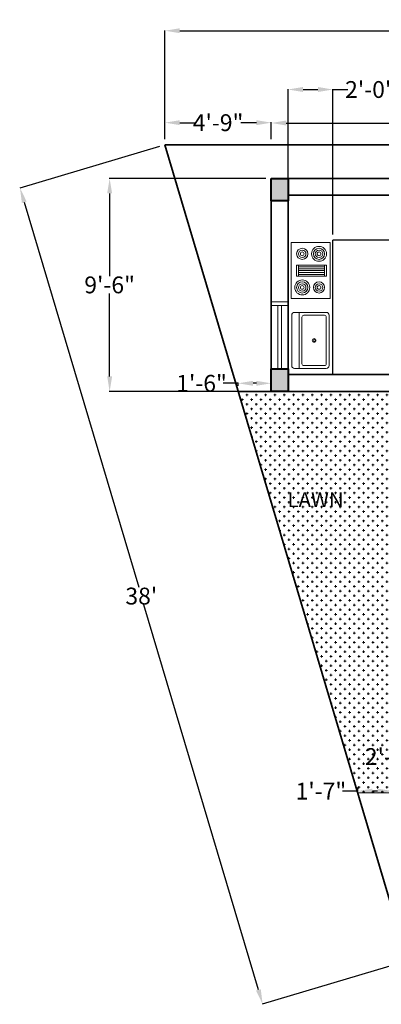
# Model space of a CAD drawing. Units: inches. Extents: x 411 to 983, y 289 to 833.
# Tile 1 of 3: x 411 to 605, y 306 to 833. Entities that reach past the tile are written whole.
import ezdxf

# ---------------------------------------------------------------- set-up
doc = ezdxf.new("R2010")
doc.units = ezdxf.units.IN
doc.header["$MEASUREMENT"] = 0
for name, color, linetype, lineweight in [('A-ANNO-DIMS', 2, 'Continuous', 18), ('A-AREA-IDEN', 7, 'Continuous', 25), ('A-COLS', 18, 'Continuous', 40), ('A-EQPM', 8, 'Continuous', 18), ('A-FLOR-CASE', 2, 'Continuous', 25), ('A-FLOR-FIXT', 9, 'Continuous', 18), ('A-GLAZ', 4, 'Continuous', 18), ('A-WALL', 4, 'Continuous', 35), ('C-PROP', 4, 'Continuous', 35), ('L-PLNT', 4, 'Continuous', 18), ('L-PLNT-PATT', 3, 'Continuous', 13)]:
    doc.layers.add(name, color=color, linetype=linetype, lineweight=lineweight)
doc.layers.add('A-COLS-PATT', color=244, linetype='Continuous', lineweight=13, true_color=0x991b1e)
doc.styles.get("Standard").update_dxf_attribs({"font": 'arial.ttf'})
doc.dimstyles.get("Standard").update_dxf_attribs({"dimtxt": 9, "dimasz": 8, "dimexe": 0.18, "dimexo": 3, "dimgap": 0.09, "dimtad": 0, "dimtih": 1, "dimtoh": 1, "dimdec": 0, "dimzin": 0, "dimdsep": 46, "dimlunit": 3, "dimtxsty": 'Standard', "dimcen": 0.09, "dimadec": 0, "dimazin": 0, "dimtfac": 1, "dimtdec": 0, "dimtofl": 0, "dimtmove": 0, "dimatfit": 3, "dimfxl": 1, "dimtolj": 1, "dimtzin": 0, "dimarcsym": 0})

# ---------------------------------------------------------------- blocks, each defined once
blk = doc.blocks.new('*D13')
at = {"layer": 'A-ANNO-DIMS', "color": 0, "lineweight": -2, "transparency": 16777216}
for p, q in [((489.14, 769.4), (489.14, 827.65)), ((867.14, 769.4), (867.14, 827.65)), ((497.14, 827.47), (662.6, 827.47)), ((859.14, 827.47), (693.69, 827.47))]:
    blk.add_line(p, q, dxfattribs=at)
at = {"layer": 'A-ANNO-DIMS', "color": 0, "transparency": 16777216}
for points in [[(497.14, 828.81), (497.14, 826.14), (489.14, 827.47)], [(859.14, 828.81), (859.14, 826.14), (867.14, 827.47)]]:
    blk.add_solid(points, dxfattribs=at)
at = {"layer": 'Defpoints', "color": 0, "transparency": 16777216}
for p in [(489.14, 827.47), (489.14, 766.4), (867.14, 766.4)]:
    blk.add_point(p, dxfattribs=at)
at = {"layer": 'A-ANNO-DIMS', "color": 0, "transparency": 16777216, "insert": (678.14, 827.47), "char_height": 9, "attachment_point": 5}
blk.add_mtext('\\A1;31\'-6"', dxfattribs=at)
blk = doc.blocks.new('*D14')
at = {"layer": 'A-ANNO-DIMS', "color": 0, "lineweight": -2, "transparency": 16777216}
for p, q in [((546.14, 769.4), (546.14, 778.25)), ((554.14, 778.07), (685.07, 778.07)), ((847.25, 778.07), (716.32, 778.07)), ((855.25, 769.4), (855.25, 778.25))]:
    blk.add_line(p, q, dxfattribs=at)
at = {"layer": 'A-ANNO-DIMS', "color": 0, "transparency": 16777216}
for points in [[(554.14, 779.41), (554.14, 776.74), (546.14, 778.07)], [(847.25, 779.41), (847.25, 776.74), (855.25, 778.07)]]:
    blk.add_solid(points, dxfattribs=at)
at = {"layer": 'Defpoints', "color": 0, "transparency": 16777216}
for p in [(546.14, 778.07), (546.14, 766.4), (855.25, 766.4)]:
    blk.add_point(p, dxfattribs=at)
at = {"layer": 'A-ANNO-DIMS', "color": 0, "transparency": 16777216, "insert": (700.7, 778.07), "char_height": 9, "attachment_point": 5}
blk.add_mtext('\\A1;25\'-9"', dxfattribs=at)
blk = doc.blocks.new('*D15')
at = {"layer": 'A-ANNO-DIMS', "color": 0, "lineweight": -2, "transparency": 16777216}
for p, q in [((489.14, 769.4), (489.14, 778.43)), ((497.14, 778.25), (505.41, 778.25)), ((538.14, 778.25), (529.88, 778.25)), ((546.14, 769.4), (546.14, 778.43))]:
    blk.add_line(p, q, dxfattribs=at)
at = {"layer": 'A-ANNO-DIMS', "color": 0, "transparency": 16777216}
for points in [[(497.14, 779.58), (497.14, 776.92), (489.14, 778.25)], [(538.14, 779.58), (538.14, 776.92), (546.14, 778.25)]]:
    blk.add_solid(points, dxfattribs=at)
at = {"layer": 'Defpoints', "color": 0, "transparency": 16777216}
for p in [(489.14, 778.25), (489.14, 766.4), (546.14, 766.4)]:
    blk.add_point(p, dxfattribs=at)
at = {"layer": 'A-ANNO-DIMS', "color": 0, "transparency": 16777216, "insert": (517.64, 778.25), "char_height": 9, "attachment_point": 5}
blk.add_mtext('\\A1;4\'-9"', dxfattribs=at)
blk = doc.blocks.new('*D16')
at = {"layer": 'A-ANNO-DIMS', "color": 0, "lineweight": -2, "transparency": 16777216}
for p, q in [((486.27, 765.55), (411.34, 743.26)), ((413.79, 735.64), (475.12, 529.5)), ((539.23, 313.98), (477.91, 520.12)), ((616.27, 328.55), (541.34, 306.26))]:
    blk.add_line(p, q, dxfattribs=at)
at = {"layer": 'A-ANNO-DIMS', "color": 0, "transparency": 16777216}
for points in [[(415.07, 736.02), (412.52, 735.26), (411.51, 743.31)], [(540.51, 314.36), (537.95, 313.6), (541.51, 306.31)]]:
    blk.add_solid(points, dxfattribs=at)
at = {"layer": 'Defpoints', "color": 0, "transparency": 16777216}
for p in [(489.14, 766.4), (411.51, 743.31), (619.14, 329.4)]:
    blk.add_point(p, dxfattribs=at)
at = {"layer": 'A-ANNO-DIMS', "color": 0, "transparency": 16777216, "insert": (476.51, 524.81), "char_height": 9, "attachment_point": 5}
blk.add_mtext("\\A1;38'", dxfattribs=at)
blk = doc.blocks.new('*D17')
at = {"layer": 'A-ANNO-DIMS', "color": 0, "lineweight": -2, "transparency": 16777216}
for p, q in [((528.41, 638.71), (520.41, 638.71)), ((528.41, 637.4), (528.41, 638.89)), ((538.14, 638.71), (536.41, 638.71)), ((546.14, 637.4), (546.14, 638.89))]:
    blk.add_line(p, q, dxfattribs=at)
at = {"layer": 'A-ANNO-DIMS', "color": 0, "transparency": 16777216}
for points in [[(536.41, 640.04), (536.41, 637.38), (528.41, 638.71)], [(538.14, 640.04), (538.14, 637.38), (546.14, 638.71)]]:
    blk.add_solid(points, dxfattribs=at)
at = {"layer": 'Defpoints', "color": 0, "transparency": 16777216}
for p in [(528.41, 638.71), (528.41, 634.4), (546.14, 634.4)]:
    blk.add_point(p, dxfattribs=at)
at = {"layer": 'A-ANNO-DIMS', "color": 0, "transparency": 16777216, "insert": (508.78, 638.71), "char_height": 9, "attachment_point": 5}
blk.add_mtext('\\A1;1\'-6"', dxfattribs=at)
blk = doc.blocks.new('*D18')
at = {"layer": 'A-ANNO-DIMS', "color": 0, "lineweight": -2, "transparency": 16777216}
for p, q in [((592.37, 422.4), (592.37, 420.58)), ((611.14, 422.4), (611.14, 420.58)), ((592.37, 420.4), (584.37, 420.4)), ((603.14, 420.4), (600.37, 420.4))]:
    blk.add_line(p, q, dxfattribs=at)
at = {"layer": 'A-ANNO-DIMS', "color": 0, "transparency": 16777216}
for points in [[(600.37, 421.73), (600.37, 419.06), (592.37, 420.4)], [(603.14, 421.73), (603.14, 419.06), (611.14, 420.4)]]:
    blk.add_solid(points, dxfattribs=at)
at = {"layer": 'Defpoints', "color": 0, "transparency": 16777216}
for p in [(592.37, 420.4), (592.37, 419.4), (611.14, 419.4)]:
    blk.add_point(p, dxfattribs=at)
at = {"layer": 'A-ANNO-DIMS', "color": 0, "transparency": 16777216, "insert": (572.74, 420.4), "char_height": 9, "attachment_point": 5}
blk.add_mtext('\\A1;1\'-7"', dxfattribs=at)
blk = doc.blocks.new('WIN-36-POST')
for p, q in [((34, 5.5), (0, 5.5)), ((34, 0), (34, 9)), ((36, 0), (36, 9)), ((34, 3.5), (0, 3.5))]:
    blk.add_line(p, q)
blk = doc.blocks.new('*D31')
at = {"layer": 'A-ANNO-DIMS', "color": 0, "lineweight": -2, "transparency": 16777216}
for p, q in [((626.14, 453.9), (623.56, 453.9)), ((623.74, 445.9), (623.74, 443.59)), ((623.74, 431.9), (623.74, 434.22)), ((626.14, 423.9), (623.56, 423.9))]:
    blk.add_line(p, q, dxfattribs=at)
at = {"layer": 'A-ANNO-DIMS', "color": 0, "transparency": 16777216}
for points in [[(622.41, 445.9), (625.08, 445.9), (623.74, 453.9)], [(622.41, 431.9), (625.08, 431.9), (623.74, 423.9)]]:
    blk.add_solid(points, dxfattribs=at)
at = {"layer": 'Defpoints', "color": 0, "transparency": 16777216}
for p in [(623.74, 453.9), (629.14, 453.9), (629.14, 423.9)]:
    blk.add_point(p, dxfattribs=at)
at = {"layer": 'A-ANNO-DIMS', "color": 0, "transparency": 16777216, "insert": (623.74, 438.9), "char_height": 9, "attachment_point": 5}
blk.add_mtext('\\A1;2\'-6" TYP.', dxfattribs=at)
blk = doc.blocks.new('*D42')
at = {"layer": 'A-ANNO-DIMS', "color": 0, "lineweight": -2, "transparency": 16777216}
for p, q in [((543.14, 748.4), (459.36, 748.4)), ((459.54, 740.4), (459.54, 696.09)), ((459.54, 642.4), (459.54, 686.72)), ((543.14, 634.4), (459.36, 634.4))]:
    blk.add_line(p, q, dxfattribs=at)
at = {"layer": 'A-ANNO-DIMS', "color": 0, "transparency": 16777216}
for points in [[(458.21, 740.4), (460.88, 740.4), (459.54, 748.4)], [(458.21, 642.4), (460.88, 642.4), (459.54, 634.4)]]:
    blk.add_solid(points, dxfattribs=at)
at = {"layer": 'Defpoints', "color": 0, "transparency": 16777216}
for p in [(546.14, 748.4), (459.54, 634.4), (546.14, 634.4)]:
    blk.add_point(p, dxfattribs=at)
at = {"layer": 'A-ANNO-DIMS', "color": 0, "transparency": 16777216, "insert": (459.54, 691.4), "char_height": 9, "attachment_point": 5}
blk.add_mtext('\\A1;9\'-6"', dxfattribs=at)
blk = doc.blocks.new('*D44')
at = {"layer": 'A-ANNO-DIMS', "color": 0, "lineweight": -2, "transparency": 16777216}
for p, q in [((555.14, 742.4), (555.14, 796.18)), ((563.14, 796), (571.14, 796)), ((579.14, 718.4), (579.14, 796.18)), ((579.14, 796), (587.14, 796))]:
    blk.add_line(p, q, dxfattribs=at)
at = {"layer": 'A-ANNO-DIMS', "color": 0, "transparency": 16777216}
for points in [[(563.14, 797.34), (563.14, 794.67), (555.14, 796)], [(571.14, 797.34), (571.14, 794.67), (579.14, 796)]]:
    blk.add_solid(points, dxfattribs=at)
at = {"layer": 'Defpoints', "color": 0, "transparency": 16777216}
for p in [(579.14, 796), (555.14, 739.4), (579.14, 715.4)]:
    blk.add_point(p, dxfattribs=at)
at = {"layer": 'A-ANNO-DIMS', "color": 0, "transparency": 16777216, "insert": (599.27, 796), "char_height": 9, "attachment_point": 5}
blk.add_mtext('\\A1;2\'-0"', dxfattribs=at)

msp = doc.modelspace()

# ---------------------------------------------------------------- hatches: boundary and pattern name
at = {"layer": 'A-COLS-PATT'}
h = msp.add_hatch(color=256, dxfattribs=at)
h.dxf.hatch_style = 1
h.paths.add_polyline_path([(625.14, 347.4), (625.14, 356.4), (615.14, 356.4), (615.14, 347.4)])
h.paths.add_polyline_path([(740.14, 347.4), (740.14, 356.4), (730.14, 356.4), (730.14, 347.4)])
h.paths.add_polyline_path([(740.14, 419.4), (749.14, 419.4), (749.14, 431.4), (740.14, 431.4)])
h.paths.add_polyline_path([(611.14, 419.4), (620.14, 419.4), (620.14, 431.4), (611.14, 431.4)])
h.paths.add_polyline_path([(846.14, 419.4), (855.14, 419.4), (855.14, 431.4), (846.14, 431.4)])
h.paths.add_polyline_path([(855.14, 612.4), (846.14, 612.4), (846.14, 600.4), (855.14, 600.4)])
h.paths.add_polyline_path([(744.14, 612.4), (735.14, 612.4), (735.14, 600.4), (744.14, 600.4)])
h.paths.add_polyline_path([(546.14, 634.4), (555.14, 634.4), (555.14, 646.4), (546.14, 646.4)])
h.paths.add_polyline_path([(555.14, 748.4), (546.14, 748.4), (546.14, 736.4), (555.14, 736.4)])
h.paths.add_polyline_path([(744.14, 748.4), (732.14, 748.4), (732.14, 739.4), (744.14, 739.4)])
h.paths.add_polyline_path([(855.14, 748.4), (846.14, 748.4), (846.14, 736.4), (855.14, 736.4)])
at = {"layer": 'L-PLNT-PATT'}
h = msp.add_hatch(dxfattribs=at)
h.set_pattern_fill('CROSS', color=256, scale=10)
h.paths.add_polyline_path([(611.14, 598.4), (611.14, 601.4), (611.14, 634.4), (528.41, 634.4), (592.37, 419.4), (611.14, 419.4), (611.14, 431.4)])
h.paths.add_polyline_path([(552.04, 568.07), (588.33, 568.07), (588.33, 584.55), (552.04, 584.55)], flags=24)

# ---------------------------------------------------------------- linework, layer by layer
at = {"layer": 'A-COLS'}
for points in [[(546.14, 748.4), (555.14, 748.4), (555.14, 736.4), (546.14, 736.4)], [(546.14, 646.4), (555.14, 646.4), (555.14, 634.4), (546.14, 634.4)]]:
    msp.add_lwpolyline(points, close=True, dxfattribs=at)
at = {"layer": 'A-EQPM'}
for p, q in [((556.73, 714.03), (577.73, 714.03)), ((556.73, 684.03), (556.73, 714.03)), ((577.73, 714.03), (577.73, 684.03)), ((559.73, 702.03), (575.73, 702.03)), ((559.73, 696.03), (559.73, 702.03)), ((560.73, 696.03), (560.73, 702.03)), ((574.73, 702.03), (574.73, 696.03)), ((575.73, 702.03), (575.73, 696.03)), ((575.73, 696.03), (559.73, 696.03)), ((560.73, 701.03), (574.73, 701.03)), ((574.73, 700.03), (560.73, 700.03)), ((560.73, 699.03), (574.73, 699.03)), ((574.73, 698.03), (560.73, 698.03)), ((560.73, 697.03), (574.73, 697.03)), ((577.73, 684.03), (556.73, 684.03))]:
    msp.add_line(p, q, dxfattribs=at)
for centre, radius in [((571.73, 708.03), 4), ((562.73, 708.03), 3), ((562.73, 708.03), 2), ((562.73, 708.03), 1), ((571.73, 708.03), 3), ((571.73, 708.03), 2), ((571.73, 708.03), 1), ((562.73, 690.03), 4), ((562.73, 690.03), 3), ((562.73, 690.03), 2), ((562.73, 690.03), 1), ((571.73, 690.03), 3), ((571.73, 690.03), 2), ((571.73, 690.03), 1)]:
    msp.add_circle(centre, radius, dxfattribs=at)
at = {"layer": 'A-FLOR-CASE'}
for p in [(688.14, 715.4), (579.14, 643.4)]:
    msp.add_line(p, (579.14, 715.4), dxfattribs=at)
at = {"layer": 'A-FLOR-FIXT'}
msp.add_line((561.1, 646.68), (561.1, 676.68), dxfattribs=at)
for points in [[(557.1, 648.18), (557.1, 675.18)], [(558.6, 676.68), (575.6, 676.68)], [(563.6, 675.18), (574.6, 675.18)], [(577.1, 675.18), (577.1, 648.18)], [(562.6, 649.18), (562.6, 674.18)], [(575.6, 674.18), (575.6, 649.18)], [(575.6, 646.68), (558.6, 646.68)], [(574.6, 648.18), (563.6, 648.18)]]:
    msp.add_lwpolyline(points, dxfattribs=at)
for radius in [1, 0.5]:
    msp.add_circle((569.1, 661.68), radius, dxfattribs=at)
for centre, radius, start, end in [((558.6, 675.18), 1.5, 90, 180), ((563.6, 674.18), 1, 90, 180), ((574.6, 674.18), 1, 0, 90), ((575.6, 675.18), 1.5, 0, 90), ((563.6, 649.18), 1, 180, 270), ((574.6, 649.18), 1, 270, 0), ((558.6, 648.18), 1.5, 180, 270), ((575.6, 648.18), 1.5, 270, 0)]:
    msp.add_arc(centre, radius, start, end, dxfattribs=at)
at = {"layer": 'A-WALL'}
for p, q in [((855.14, 748.4), (546.14, 748.4)), ((546.14, 634.4), (546.14, 748.4)), ((555.14, 643.4), (555.14, 739.4)), ((688.14, 739.4), (555.14, 739.4)), ((632.14, 643.4), (555.14, 643.4)), ((611.14, 634.4), (528.41, 634.4))]:
    msp.add_line(p, q, dxfattribs=at)
at = {"layer": 'C-PROP'}
for p, q in [((867.14, 766.4), (489.14, 766.4)), ((489.14, 766.4), (619.14, 329.4))]:
    msp.add_line(p, q, dxfattribs=at)
at = {"layer": 'L-PLNT'}
msp.add_line((611.14, 419.4), (592.37, 419.4), dxfattribs=at)

# ---------------------------------------------------------------- block references
at = {"layer": 'A-GLAZ', "rotation": 90.00000000000003}
msp.add_blockref('WIN-36-POST', (555.14, 646.4), dxfattribs=at)

# ---------------------------------------------------------------- texts
at = {"layer": 'A-AREA-IDEN', "insert": (554.86, 580.43), "char_height": 8, "attachment_point": 1}
msp.add_mtext_dynamic_manual_height_columns('LAWN', width=69.531, gutter_width=1, heights=[0], dxfattribs=at)

# ---------------------------------------------------------------- dimensions: what is measured, and where the dimension line sits
at = {"layer": 'A-ANNO-DIMS'}
for base, p1, p2, override, picture, middle in [((489.14, 827.47), (867.14, 766.4), (489.14, 766.4), {"dimclrd": 0, "dimclre": 0, "dimclrt": 0}, '*D13', (678.14, 827.47)), ((579.14, 796), (555.14, 739.4), (579.14, 715.4), {"dimdec": 1, "dimlfac": 1, "dimrnd": 0, "dimzin": 1, "dimdsep": 46, "dimlunit": 4, "dimfrac": 2}, '*D44', (599.27, 796)), ((489.14, 778.25), (546.14, 766.4), (489.14, 766.4), {"dimclrd": 0, "dimclre": 0, "dimclrt": 0}, '*D15', (517.64, 778.25)), ((546.14, 778.07), (855.25, 766.4), (546.14, 766.4), {"dimclrd": 0, "dimclre": 0, "dimclrt": 0}, '*D14', (700.7, 778.07)), ((528.41, 638.71), (546.14, 634.4), (528.41, 634.4), {"dimclrd": 0, "dimclre": 0, "dimclrt": 0}, '*D17', (508.78, 638.71)), ((592.37, 420.4), (611.14, 419.4), (592.37, 419.4), {"dimclrd": 0, "dimclre": 0, "dimclrt": 0}, '*D18', (572.74, 420.4))]:
    dim = msp.add_linear_dim(base=base, p1=p1, p2=p2, dimstyle='Standard', override=override, dxfattribs=at)
    dim.commit()
    dim.dimension.update_dxf_attribs({"geometry": picture, "text_midpoint": middle})
dim = msp.add_aligned_dim(p1=(619.14, 329.4), p2=(489.14, 766.4), distance=80.99, dimstyle='Standard', override={"dimclrd": 0, "dimclre": 0, "dimclrt": 0}, dxfattribs=at)
dim.commit()
dim.dimension.update_dxf_attribs({"geometry": '*D16', "text_midpoint": (476.51, 524.81)})
dim = msp.add_linear_dim(base=(459.54, 634.4), p1=(546.14, 748.4), p2=(546.14, 634.4), angle=90, dimstyle='Standard', override={"dimdec": 1, "dimlfac": 1, "dimrnd": 0, "dimzin": 1, "dimdsep": 46, "dimlunit": 4, "dimfrac": 2}, dxfattribs=at)
dim.commit()
dim.dimension.update_dxf_attribs({"geometry": '*D42', "text_midpoint": (459.54, 691.4)})
dim = msp.add_linear_dim(base=(623.74, 453.9), p1=(629.14, 423.9), p2=(629.14, 453.9), angle=90, text='<> TYP.', dimstyle='Standard', override={"dimdec": 1, "dimlfac": 1, "dimrnd": 0, "dimzin": 1, "dimdsep": 46, "dimlunit": 4, "dimfrac": 2}, dxfattribs=at)
dim.commit()
dim.dimension.update_dxf_attribs({"geometry": '*D31', "text_midpoint": (623.74, 438.9)})

doc.saveas('drawing.dxf')
